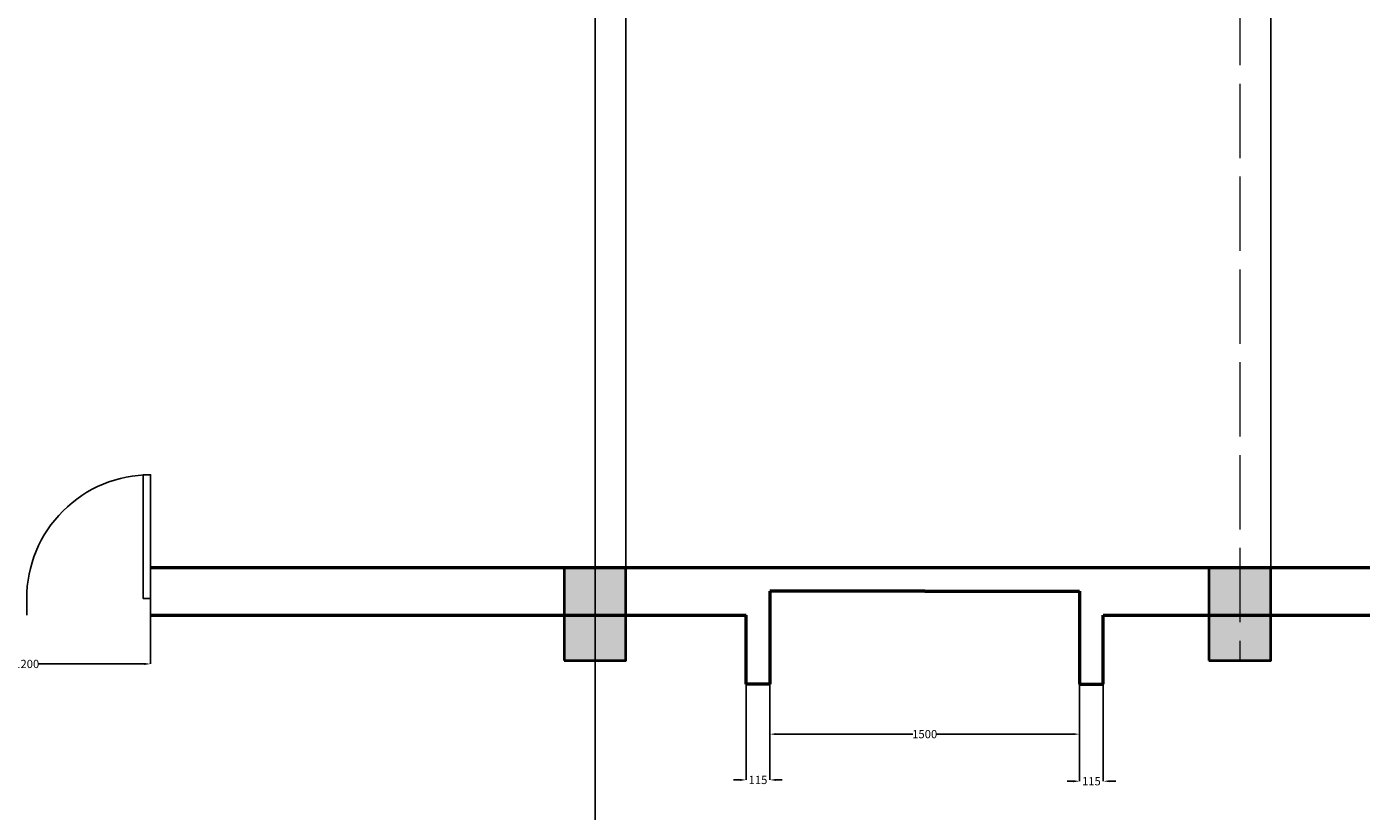
# Model space of a CAD drawing. Units: millimetres. Extents: x -17156 to 39375, y -45872 to -24892.
# Tile 6 of 12: x -5337 to 1128, y -41514 to -37711. Entities that reach past the tile are written whole.
import ezdxf

# ---------------------------------------------------------------- set-up
doc = ezdxf.new("R2010")
doc.units = ezdxf.units.MM
doc.header["$MEASUREMENT"] = 0
doc.linetypes.add('ACAD_ISO02W100', pattern=[15, 12, -3])
for name, color, linetype, lineweight in [('A-ANNO-DIMS', 2, 'Continuous', 18), ('A-COLS', 7, 'Continuous', 40), ('DOORS', 6, 'Continuous', 25), ('S-BEAM-OVHD', 8, 'ACAD_ISO02W100', 18), ('WALLS', 5, 'Continuous', 50)]:
    doc.layers.add(name, color=color, linetype=linetype, lineweight=lineweight)
doc.styles.get("Standard").update_dxf_attribs({"font": 'arial.ttf'})
doc.dimstyles.get("Standard").update_dxf_attribs({"dimtxt": 40, "dimasz": 30.18, "dimexe": 0, "dimexo": 0.0625, "dimgap": 0.09, "dimtad": 0, "dimtih": 1, "dimtoh": 1, "dimdec": 0, "dimzin": 0, "dimdsep": 46, "dimtxsty": 'Standard', "dimcen": 0.09, "dimadec": 0, "dimazin": 0, "dimtfac": 1, "dimtdec": 0, "dimtofl": 0, "dimtmove": 0, "dimatfit": 3, "dimfxl": 1, "dimtolj": 1, "dimtzin": 0, "dimarcsym": 0})

# ---------------------------------------------------------------- blocks, each defined once
blk = doc.blocks.new('*U7')
for p, q in [((0, 0), (0, 100)), ((750, 0), (750, 100))]:
    blk.add_line(p, q)
blk.add_lwpolyline([(0, 0), (0, -750), (43.75, -750), (43.75, 0)], close=True)
blk.add_arc((0, 0), 750, 270, 0)
blk = doc.blocks.new('*D94')
at = {"layer": 'A-ANNO-DIMS', "color": 0, "lineweight": -2, "transparency": 16777216}
for p, q in [((-5937.3, -40562.9), (-5937.3, -40799.8)), ((-4737.3, -40562.9), (-4737.3, -40799.8)), ((-5907.2, -40799.8), (-5395.2, -40799.8)), ((-4767.5, -40799.8), (-5279.5, -40799.8))]:
    blk.add_line(p, q, dxfattribs=at)
at = {"layer": 'A-ANNO-DIMS', "color": 0, "lineweight": 100, "transparency": 16777216}
for points in [[(-5907.2, -40794.7), (-5907.2, -40804.8), (-5937.3, -40799.8)], [(-4767.5, -40794.7), (-4767.5, -40804.8), (-4737.3, -40799.8)]]:
    blk.add_solid(points, dxfattribs=at)
at = {"layer": 'Defpoints', "color": 0, "lineweight": 100, "transparency": 16777216}
for p in [(-5937.3, -40562.8), (-4737.3, -40562.8), (-5937.3, -40799.8)]:
    blk.add_point(p, dxfattribs=at)
at = {"layer": 'A-ANNO-DIMS', "color": 0, "transparency": 16777216, "insert": (-5337.3, -40799.8), "char_height": 40, "attachment_point": 5}
blk.add_mtext('\\A1;1200', dxfattribs=at)
blk = doc.blocks.new('*D95')
at = {"layer": 'A-ANNO-DIMS', "color": 0, "lineweight": -2, "transparency": 16777216}
for p, q in [((-1852.3, -40897.9), (-1852.3, -41361.9)), ((-1737.3, -40897.9), (-1737.3, -41361.9)), ((-1882.5, -41361.9), (-1912.7, -41361.9)), ((-1707.2, -41361.9), (-1677, -41361.9))]:
    blk.add_line(p, q, dxfattribs=at)
at = {"layer": 'A-ANNO-DIMS', "color": 0, "lineweight": 100, "transparency": 16777216}
for points in [[(-1882.5, -41356.9), (-1882.5, -41366.9), (-1852.3, -41361.9)], [(-1707.2, -41356.9), (-1707.2, -41366.9), (-1737.3, -41361.9)]]:
    blk.add_solid(points, dxfattribs=at)
at = {"layer": 'Defpoints', "color": 0, "lineweight": 100, "transparency": 16777216}
for p in [(-1852.3, -40897.8), (-1737.3, -40897.8), (-1852.3, -41361.9)]:
    blk.add_point(p, dxfattribs=at)
at = {"layer": 'A-ANNO-DIMS', "color": 0, "transparency": 16777216, "insert": (-1794.8, -41361.9), "char_height": 40, "attachment_point": 5}
blk.add_mtext('\\A1;115', dxfattribs=at)
blk = doc.blocks.new('*D96')
at = {"layer": 'A-ANNO-DIMS', "color": 0, "lineweight": -2, "transparency": 16777216}
for p, q in [((-237.3, -40897.9), (-237.3, -41368.2)), ((-122.3, -40897.9), (-122.3, -41368.2)), ((-267.5, -41368.2), (-297.7, -41368.2)), ((-92.2, -41368.2), (-62, -41368.2))]:
    blk.add_line(p, q, dxfattribs=at)
at = {"layer": 'A-ANNO-DIMS', "color": 0, "lineweight": 100, "transparency": 16777216}
for points in [[(-267.5, -41363.1), (-267.5, -41373.2), (-237.3, -41368.2)], [(-92.2, -41363.1), (-92.2, -41373.2), (-122.3, -41368.2)]]:
    blk.add_solid(points, dxfattribs=at)
at = {"layer": 'Defpoints', "color": 0, "lineweight": 100, "transparency": 16777216}
for p in [(-237.3, -40897.8), (-122.3, -40897.8), (-122.3, -41368.2)]:
    blk.add_point(p, dxfattribs=at)
at = {"layer": 'A-ANNO-DIMS', "color": 0, "transparency": 16777216, "insert": (-179.8, -41368.2), "char_height": 40, "attachment_point": 5}
blk.add_mtext('\\A1;115', dxfattribs=at)
blk = doc.blocks.new('*D97')
at = {"layer": 'A-ANNO-DIMS', "color": 0, "lineweight": -2, "transparency": 16777216}
for p, q in [((-1737.3, -40897.9), (-1737.3, -41139.9)), ((-237.3, -40897.9), (-237.3, -41139.9)), ((-1707.2, -41139.9), (-1045.2, -41139.9)), ((-267.5, -41139.9), (-929.5, -41139.9))]:
    blk.add_line(p, q, dxfattribs=at)
at = {"layer": 'A-ANNO-DIMS', "color": 0, "lineweight": 100, "transparency": 16777216}
for points in [[(-1707.2, -41134.9), (-1707.2, -41144.9), (-1737.3, -41139.9)], [(-267.5, -41134.9), (-267.5, -41144.9), (-237.3, -41139.9)]]:
    blk.add_solid(points, dxfattribs=at)
at = {"layer": 'Defpoints', "color": 0, "lineweight": 100, "transparency": 16777216}
for p in [(-1737.3, -40897.8), (-237.3, -40897.8), (-1737.3, -41139.9)]:
    blk.add_point(p, dxfattribs=at)
at = {"layer": 'A-ANNO-DIMS', "color": 0, "transparency": 16777216, "insert": (-987.3, -41139.9), "char_height": 40, "attachment_point": 5}
blk.add_mtext('\\A1;1500', dxfattribs=at)
blk = doc.blocks.new('COL-450x300')
h = blk.add_hatch(color=256)
h.dxf.hatch_style = 1
h.paths.add_polyline_path([(0, 300), (0, 0), (450, 0), (450, 300)])
blk.add_lwpolyline([(0, 300), (0, 0), (450, 0), (450, 300)], close=True)
blk = doc.blocks.new('*D145')
at = {"layer": 'A-ANNO-DIMS', "color": 0, "lineweight": -2, "transparency": 16777216}
for p, q in [((-6237.4, -27247.8), (-17080.3, -27247.8)), ((-17080.3, -27278), (-17080.3, -35684.8)), ((-17080.3, -44132.7), (-17080.3, -35725.9)), ((-2887.4, -44162.8), (-17080.3, -44162.8))]:
    blk.add_line(p, q, dxfattribs=at)
at = {"layer": 'A-ANNO-DIMS', "color": 0, "lineweight": 100, "transparency": 16777216}
for points in [[(-17085.4, -27278), (-17075.3, -27278), (-17080.3, -27247.8)], [(-17085.4, -44132.7), (-17075.3, -44132.7), (-17080.3, -44162.8)]]:
    blk.add_solid(points, dxfattribs=at)
at = {"layer": 'Defpoints', "color": 0, "lineweight": 100, "transparency": 16777216}
for p in [(-6237.3, -27247.8), (-17080.3, -44162.8), (-2887.3, -44162.8)]:
    blk.add_point(p, dxfattribs=at)
at = {"layer": 'A-ANNO-DIMS', "color": 0, "transparency": 16777216, "insert": (-17080.3, -35705.3), "char_height": 40, "attachment_point": 5}
blk.add_mtext('\\A1;16915', dxfattribs=at)
blk = doc.blocks.new('*D151')
at = {"layer": 'A-ANNO-DIMS', "color": 0, "lineweight": -2, "transparency": 16777216}
for p, q in [((-6122.3, -42547.8), (-6122.3, -25564.8)), ((-6092.2, -25564.8), (-4413.2, -25564.8)), ((-2614.5, -25564.8), (-4293.5, -25564.8)), ((-2584.3, -42547.8), (-2584.3, -25564.8))]:
    blk.add_line(p, q, dxfattribs=at)
at = {"layer": 'A-ANNO-DIMS', "color": 0, "lineweight": 100, "transparency": 16777216}
for points in [[(-6092.2, -25559.8), (-6092.2, -25569.9), (-6122.3, -25564.8)], [(-2614.5, -25559.8), (-2614.5, -25569.9), (-2584.3, -25564.8)]]:
    blk.add_solid(points, dxfattribs=at)
at = {"layer": 'Defpoints', "color": 0, "lineweight": 100, "transparency": 16777216}
for p in [(-2584.3, -25564.8), (-6122.3, -42547.8), (-2584.3, -42547.8)]:
    blk.add_point(p, dxfattribs=at)
at = {"layer": 'A-ANNO-DIMS', "color": 0, "transparency": 16777216, "insert": (-4353.3, -25564.8), "char_height": 40, "attachment_point": 5}
blk.add_mtext('\\A1;3538', dxfattribs=at)
blk = doc.blocks.new('*D152')
at = {"layer": 'A-ANNO-DIMS', "color": 0, "lineweight": -2, "transparency": 16777216}
for p, q in [((-2434.3, -40332.8), (-2434.3, -25564.8)), ((-2404.2, -25564.8), (-932.1, -25564.8)), ((659.5, -25564.8), (-812.6, -25564.8)), ((689.7, -40332.8), (689.7, -25564.8))]:
    blk.add_line(p, q, dxfattribs=at)
at = {"layer": 'A-ANNO-DIMS', "color": 0, "lineweight": 100, "transparency": 16777216}
for points in [[(-2404.2, -25559.8), (-2404.2, -25569.9), (-2434.3, -25564.8)], [(659.5, -25559.8), (659.5, -25569.9), (689.7, -25564.8)]]:
    blk.add_solid(points, dxfattribs=at)
at = {"layer": 'Defpoints', "color": 0, "lineweight": 100, "transparency": 16777216}
for p in [(689.7, -25564.8), (-2434.3, -40332.8), (689.7, -40332.8)]:
    blk.add_point(p, dxfattribs=at)
at = {"layer": 'A-ANNO-DIMS', "color": 0, "transparency": 16777216, "insert": (-872.3, -25564.8), "char_height": 40, "attachment_point": 5}
blk.add_mtext('\\A1;3124', dxfattribs=at)

msp = doc.modelspace()

# ---------------------------------------------------------------- linework, layer by layer
at = {"layer": 'S-BEAM-OVHD', "ltscale": 30}
for p, q in [((-2584.35, -34837.85), (-2584.35, -40782.85)), ((539.65, -34837.85), (539.65, -40782.85))]:
    msp.add_line(p, q, dxfattribs=at)
at = {"layer": 'WALLS'}
for p, q in [((-4737.35, -40332.85), (2762.65, -40332.85)), ((-987.35, -40447.85), (-1737.35, -40447.85)), ((-1737.35, -40447.85), (-1737.35, -40897.85)), ((-987.35, -40447.85), (-237.35, -40447.85)), ((-237.35, -40447.85), (-237.35, -40897.85)), ((-4737.35, -40562.85), (-1852.35, -40562.85)), ((-1852.35, -40897.85), (-1852.35, -40562.85)), ((-122.35, -40897.85), (-122.35, -40562.85)), ((-122.35, -40562.85), (2762.65, -40562.85)), ((-1737.35, -40897.85), (-1852.35, -40897.85)), ((-237.35, -40897.85), (-122.35, -40897.85))]:
    msp.add_line(p, q, dxfattribs=at)

# ---------------------------------------------------------------- block references
at = {"layer": 'A-COLS'}
for p, rotation in [((-2434.35, -40782.85), 90.00000000000134), ((689.65, -40782.85), 90.00000000000126), ((689.65, -40782.85), 90.00000000000126)]:
    msp.add_blockref('COL-450x300', p, dxfattribs=dict(at, rotation=rotation))
at = {"layer": 'DOORS', "xscale": 0.8, "yscale": 0.8, "zscale": 0.8, "rotation": 180}
msp.add_blockref('*U7', (-4737.35, -40482.85), dxfattribs=at)

# ---------------------------------------------------------------- dimensions: what is measured, and where the dimension line sits
at = {"layer": 'A-ANNO-DIMS'}
for base, p1, p2, override, picture, middle in [((-2584.35, -25564.85), (-6122.35, -42547.85), (-2584.35, -42547.85), {"dimdec": 0, "dimlfac": 1, "dimrnd": 0, "dimzin": 0, "dimdsep": 46, "dimlunit": 2}, '*D151', (-4353.35, -25564.85)), ((689.65, -25564.85), (-2434.35, -40332.85), (689.65, -40332.85), {"dimdec": 0, "dimlfac": 1, "dimrnd": 0, "dimzin": 0, "dimdsep": 46, "dimlunit": 2}, '*D152', (-872.35, -25564.85)), ((-5937.35, -40799.77), (-4737.35, -40562.85), (-5937.35, -40562.85), {"dimclrd": 0, "dimclre": 0, "dimclrt": 0}, '*D94', (-5337.35, -40799.77)), ((-1852.35, -41361.89), (-1737.35, -40897.85), (-1852.35, -40897.85), {"dimclrd": 0, "dimclre": 0, "dimclrt": 0}, '*D95', (-1794.85, -41361.89)), ((-1737.35, -41139.89), (-237.35, -40897.85), (-1737.35, -40897.85), {"dimclrd": 0, "dimclre": 0, "dimclrt": 0}, '*D97', (-987.35, -41139.89)), ((-122.35, -41368.16), (-237.35, -40897.85), (-122.35, -40897.85), {"dimclrd": 0, "dimclre": 0, "dimclrt": 0}, '*D96', (-179.85, -41368.16))]:
    dim = msp.add_linear_dim(base=base, p1=p1, p2=p2, dimstyle='Standard', override=override, dxfattribs=at)
    dim.commit()
    dim.dimension.update_dxf_attribs({"geometry": picture, "text_midpoint": middle})
dim = msp.add_linear_dim(base=(-17080.35, -44162.85), p1=(-6237.35, -27247.85), p2=(-2887.35, -44162.85), angle=90, dimstyle='Standard', override={"dimdec": 0, "dimlfac": 1, "dimrnd": 0, "dimzin": 0, "dimdsep": 46, "dimlunit": 2}, dxfattribs=at)
dim.commit()
dim.dimension.update_dxf_attribs({"geometry": '*D145', "text_midpoint": (-17080.35, -35705.35)})

doc.saveas('drawing.dxf')
